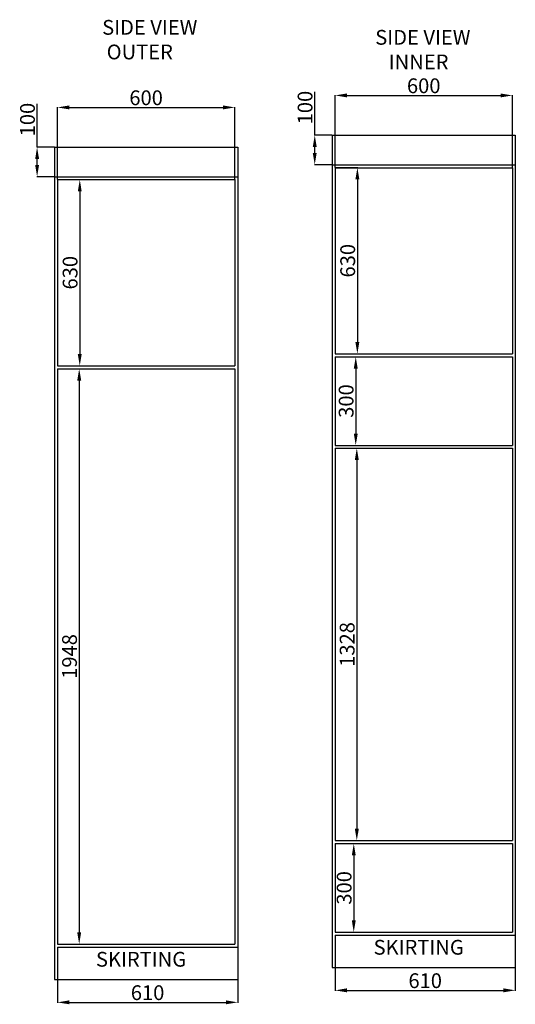
# Model space of a CAD drawing. Units: millimetres. Extents: x 46070 to 59439, y 6883 to 14761.
# Tile 4 of 5: x 56815 to 58493, y 7101 to 10434. Entities that reach past the tile are written whole.
import ezdxf

# ---------------------------------------------------------------- set-up
doc = ezdxf.new("R2010")
doc.units = ezdxf.units.MM
for name, color, linetype, lineweight in [('A-ANNO-DIMS', 2, 'Continuous', 18), ('A-ANNO-TEXT', 7, 'Continuous', 18), ('A-ELEV', 7, 'Continuous', 25)]:
    doc.layers.add(name, color=color, linetype=linetype, lineweight=lineweight)
doc.styles.get("Standard").update_dxf_attribs({"font": 'arial.ttf'})
doc.dimstyles.new('ISO-25', dxfattribs={"dimtxt": 50, "dimasz": 40, "dimexe": 1.25, "dimexo": 0.625, "dimtad": 1, "dimtxsty": 'Standard', "dimcen": 2.5, "dimadec": 0, "dimazin": 0, "dimtfac": 1, "dimtmove": 0, "dimatfit": 3, "dimfxl": 1, "dimarcsym": 0})

# ---------------------------------------------------------------- blocks, each defined once
blk = doc.blocks.new('*D68')
at = {"layer": 'A-ANNO-DIMS', "color": 0, "lineweight": -2, "transparency": 16777216}
for p, q in [((57883.3, 7644.7), (57947.2, 7644.7)), ((57945.9, 7604.7), (57945.9, 7384.7)), ((57883.3, 7344.7), (57947.2, 7344.7))]:
    blk.add_line(p, q, dxfattribs=at)
at = {"layer": 'A-ANNO-DIMS', "color": 0, "transparency": 16777216}
for points in [[(57939.3, 7604.7), (57952.6, 7604.7), (57945.9, 7644.7)], [(57939.3, 7384.7), (57952.6, 7384.7), (57945.9, 7344.7)]]:
    blk.add_solid(points, dxfattribs=at)
at = {"layer": 'Defpoints', "color": 0, "transparency": 16777216}
for p in [(57882.7, 7644.7), (57882.7, 7344.7), (57945.9, 7344.7)]:
    blk.add_point(p, dxfattribs=at)
at = {"layer": 'A-ANNO-DIMS', "color": 0, "transparency": 16777216, "insert": (57919.8, 7494.7), "char_height": 50, "attachment_point": 5, "rotation": 90}
blk.add_mtext('300', dxfattribs=at)
blk = doc.blocks.new('*D69')
at = {"layer": 'A-ANNO-DIMS', "color": 0, "lineweight": -2, "transparency": 16777216}
for p, q in [((57883.3, 8982.7), (57957.5, 8982.7)), ((57956.2, 8942.7), (57956.2, 7694.7)), ((57883.3, 7654.7), (57957.5, 7654.7))]:
    blk.add_line(p, q, dxfattribs=at)
at = {"layer": 'A-ANNO-DIMS', "color": 0, "transparency": 16777216}
for points in [[(57949.5, 8942.7), (57962.9, 8942.7), (57956.2, 8982.7)], [(57949.5, 7694.7), (57962.9, 7694.7), (57956.2, 7654.7)]]:
    blk.add_solid(points, dxfattribs=at)
at = {"layer": 'Defpoints', "color": 0, "transparency": 16777216}
for p in [(57882.7, 8982.7), (57882.7, 7654.7), (57956.2, 7654.7)]:
    blk.add_point(p, dxfattribs=at)
at = {"layer": 'A-ANNO-DIMS', "color": 0, "transparency": 16777216, "insert": (57930, 8318.7), "char_height": 50, "attachment_point": 5, "rotation": 90}
blk.add_mtext('1328', dxfattribs=at)
blk = doc.blocks.new('*D70')
at = {"layer": 'A-ANNO-DIMS', "color": 0, "lineweight": -2, "transparency": 16777216}
for p, q in [((57883.3, 9292.7), (57953.9, 9292.7)), ((57952.6, 9252.7), (57952.6, 9032.7)), ((57883.3, 8992.7), (57953.9, 8992.7))]:
    blk.add_line(p, q, dxfattribs=at)
at = {"layer": 'A-ANNO-DIMS', "color": 0, "transparency": 16777216}
for points in [[(57946, 9252.7), (57959.3, 9252.7), (57952.6, 9292.7)], [(57946, 9032.7), (57959.3, 9032.7), (57952.6, 8992.7)]]:
    blk.add_solid(points, dxfattribs=at)
at = {"layer": 'Defpoints', "color": 0, "transparency": 16777216}
for p in [(57882.7, 9292.7), (57882.7, 8992.7), (57952.6, 8992.7)]:
    blk.add_point(p, dxfattribs=at)
at = {"layer": 'A-ANNO-DIMS', "color": 0, "transparency": 16777216, "insert": (57926.5, 9142.7), "char_height": 50, "attachment_point": 5, "rotation": 90}
blk.add_mtext('300', dxfattribs=at)
blk = doc.blocks.new('*D71')
at = {"layer": 'A-ANNO-DIMS', "color": 0, "lineweight": -2, "transparency": 16777216}
for p, q in [((57883.3, 9932.7), (57959.3, 9932.7)), ((57958.1, 9892.7), (57958.1, 9342.7)), ((57883.3, 9302.7), (57959.3, 9302.7))]:
    blk.add_line(p, q, dxfattribs=at)
at = {"layer": 'A-ANNO-DIMS', "color": 0, "transparency": 16777216}
for points in [[(57951.4, 9892.7), (57964.8, 9892.7), (57958.1, 9932.7)], [(57951.4, 9342.7), (57964.8, 9342.7), (57958.1, 9302.7)]]:
    blk.add_solid(points, dxfattribs=at)
at = {"layer": 'Defpoints', "color": 0, "transparency": 16777216}
for p in [(57882.7, 9932.7), (57882.7, 9302.7), (57958.1, 9302.7)]:
    blk.add_point(p, dxfattribs=at)
at = {"layer": 'A-ANNO-DIMS', "color": 0, "transparency": 16777216, "insert": (57931.9, 9617.7), "char_height": 50, "attachment_point": 5, "rotation": 90}
blk.add_mtext('630', dxfattribs=at)
blk = doc.blocks.new('*D72')
at = {"layer": 'A-ANNO-DIMS', "color": 0, "lineweight": -2, "transparency": 16777216}
for p, q in [((57813.8, 10042.7), (57813.8, 10189.5)), ((57872.1, 10042.7), (57812.5, 10042.7)), ((57813.8, 9982.7), (57813.8, 10002.7)), ((57872.1, 9942.7), (57812.5, 9942.7))]:
    blk.add_line(p, q, dxfattribs=at)
at = {"layer": 'A-ANNO-DIMS', "color": 0, "transparency": 16777216}
for points in [[(57807.1, 10002.7), (57820.4, 10002.7), (57813.8, 10042.7)], [(57807.1, 9982.7), (57820.4, 9982.7), (57813.8, 9942.7)]]:
    blk.add_solid(points, dxfattribs=at)
at = {"layer": 'Defpoints', "color": 0, "transparency": 16777216}
for p in [(57813.8, 10042.7), (57872.7, 10042.7), (57872.7, 9942.7)]:
    blk.add_point(p, dxfattribs=at)
at = {"layer": 'A-ANNO-DIMS', "color": 0, "transparency": 16777216, "insert": (57787.6, 10136.1), "char_height": 50, "attachment_point": 5, "rotation": 90}
blk.add_mtext('100', dxfattribs=at)
blk = doc.blocks.new('*D73')
at = {"layer": 'A-ANNO-DIMS', "color": 0, "lineweight": -2, "transparency": 16777216}
for p, q in [((57882.7, 7334.1), (57882.7, 7146.6)), ((58492.7, 7334.1), (58492.7, 7146.6)), ((57922.7, 7147.8), (58452.7, 7147.8))]:
    blk.add_line(p, q, dxfattribs=at)
at = {"layer": 'A-ANNO-DIMS', "color": 0, "transparency": 16777216}
for points in [[(57922.7, 7154.5), (57922.7, 7141.2), (57882.7, 7147.8)], [(58452.7, 7154.5), (58452.7, 7141.2), (58492.7, 7147.8)]]:
    blk.add_solid(points, dxfattribs=at)
at = {"layer": 'Defpoints', "color": 0, "transparency": 16777216}
for p in [(57882.7, 7334.7), (58492.7, 7334.7), (58492.7, 7147.8)]:
    blk.add_point(p, dxfattribs=at)
at = {"layer": 'A-ANNO-DIMS', "color": 0, "transparency": 16777216, "insert": (58187.7, 7174), "char_height": 50, "attachment_point": 5}
blk.add_mtext('610', dxfattribs=at)
blk = doc.blocks.new('*D74')
at = {"layer": 'A-ANNO-DIMS', "color": 0, "lineweight": -2, "transparency": 16777216}
for p, q in [((57882.7, 9933.3), (57882.7, 10178.5)), ((57922.7, 10177.2), (58442.7, 10177.2)), ((58482.7, 9933.3), (58482.7, 10178.5))]:
    blk.add_line(p, q, dxfattribs=at)
at = {"layer": 'A-ANNO-DIMS', "color": 0, "transparency": 16777216}
for points in [[(57922.7, 10183.9), (57922.7, 10170.6), (57882.7, 10177.2)], [(58442.7, 10183.9), (58442.7, 10170.6), (58482.7, 10177.2)]]:
    blk.add_solid(points, dxfattribs=at)
at = {"layer": 'Defpoints', "color": 0, "transparency": 16777216}
for p in [(58482.7, 10177.2), (57882.7, 9932.7), (58482.7, 9932.7)]:
    blk.add_point(p, dxfattribs=at)
at = {"layer": 'A-ANNO-DIMS', "color": 0, "transparency": 16777216, "insert": (58182.7, 10203.4), "char_height": 50, "attachment_point": 5}
blk.add_mtext('600', dxfattribs=at)
blk = doc.blocks.new('*D75')
at = {"layer": 'A-ANNO-DIMS', "color": 0, "lineweight": -2, "transparency": 16777216}
for p, q in [((56943.6, 9252.1), (57017.7, 9252.1)), ((57016.5, 9212.1), (57016.5, 7344.1)), ((56943.6, 7304.1), (57017.7, 7304.1))]:
    blk.add_line(p, q, dxfattribs=at)
at = {"layer": 'A-ANNO-DIMS', "color": 0, "transparency": 16777216}
for points in [[(57009.8, 9212.1), (57023.2, 9212.1), (57016.5, 9252.1)], [(57009.8, 7344.1), (57023.2, 7344.1), (57016.5, 7304.1)]]:
    blk.add_solid(points, dxfattribs=at)
at = {"layer": 'Defpoints', "color": 0, "transparency": 16777216}
for p in [(56943, 9252.1), (56943, 7304.1), (57016.5, 7304.1)]:
    blk.add_point(p, dxfattribs=at)
at = {"layer": 'A-ANNO-DIMS', "color": 0, "transparency": 16777216, "insert": (56990.3, 8278.1), "char_height": 50, "attachment_point": 5, "rotation": 90}
blk.add_mtext('1948', dxfattribs=at)
blk = doc.blocks.new('*D76')
at = {"layer": 'A-ANNO-DIMS', "color": 0, "lineweight": -2, "transparency": 16777216}
for p, q in [((56943.6, 9892.1), (57019.6, 9892.1)), ((57018.4, 9852.1), (57018.4, 9302.1)), ((56943.6, 9262.1), (57019.6, 9262.1))]:
    blk.add_line(p, q, dxfattribs=at)
at = {"layer": 'A-ANNO-DIMS', "color": 0, "transparency": 16777216}
for points in [[(57011.7, 9852.1), (57025, 9852.1), (57018.4, 9892.1)], [(57011.7, 9302.1), (57025, 9302.1), (57018.4, 9262.1)]]:
    blk.add_solid(points, dxfattribs=at)
at = {"layer": 'Defpoints', "color": 0, "transparency": 16777216}
for p in [(56943, 9892.1), (56943, 9262.1), (57018.4, 9262.1)]:
    blk.add_point(p, dxfattribs=at)
at = {"layer": 'A-ANNO-DIMS', "color": 0, "transparency": 16777216, "insert": (56992.2, 9577.1), "char_height": 50, "attachment_point": 5, "rotation": 90}
blk.add_mtext('630', dxfattribs=at)
blk = doc.blocks.new('*D77')
at = {"layer": 'A-ANNO-DIMS', "color": 0, "lineweight": -2, "transparency": 16777216}
for p, q in [((56874, 10002.1), (56874, 10148.9)), ((56932.4, 10002.1), (56872.8, 10002.1)), ((56874, 9942.1), (56874, 9962.1)), ((56932.4, 9902.1), (56872.8, 9902.1))]:
    blk.add_line(p, q, dxfattribs=at)
at = {"layer": 'A-ANNO-DIMS', "color": 0, "transparency": 16777216}
for points in [[(56867.4, 9962.1), (56880.7, 9962.1), (56874, 10002.1)], [(56867.4, 9942.1), (56880.7, 9942.1), (56874, 9902.1)]]:
    blk.add_solid(points, dxfattribs=at)
at = {"layer": 'Defpoints', "color": 0, "transparency": 16777216}
for p in [(56874, 10002.1), (56933, 10002.1), (56933, 9902.1)]:
    blk.add_point(p, dxfattribs=at)
at = {"layer": 'A-ANNO-DIMS', "color": 0, "transparency": 16777216, "insert": (56847.9, 10095.5), "char_height": 50, "attachment_point": 5, "rotation": 90}
blk.add_mtext('100', dxfattribs=at)
blk = doc.blocks.new('*D78')
at = {"layer": 'A-ANNO-DIMS', "color": 0, "lineweight": -2, "transparency": 16777216}
for p, q in [((56943, 7293.4), (56943, 7106)), ((57553, 7293.4), (57553, 7106)), ((56983, 7107.2), (57513, 7107.2))]:
    blk.add_line(p, q, dxfattribs=at)
at = {"layer": 'A-ANNO-DIMS', "color": 0, "transparency": 16777216}
for points in [[(56983, 7113.9), (56983, 7100.6), (56943, 7107.2)], [(57513, 7113.9), (57513, 7100.6), (57553, 7107.2)]]:
    blk.add_solid(points, dxfattribs=at)
at = {"layer": 'Defpoints', "color": 0, "transparency": 16777216}
for p in [(56943, 7294.1), (57553, 7294.1), (57553, 7107.2)]:
    blk.add_point(p, dxfattribs=at)
at = {"layer": 'A-ANNO-DIMS', "color": 0, "transparency": 16777216, "insert": (57248, 7133.4), "char_height": 50, "attachment_point": 5}
blk.add_mtext('610', dxfattribs=at)
blk = doc.blocks.new('*D79')
at = {"layer": 'A-ANNO-DIMS', "color": 0, "lineweight": -2, "transparency": 16777216}
for p, q in [((56943, 9892.7), (56943, 10137.9)), ((56983, 10136.6), (57503, 10136.6)), ((57543, 9892.7), (57543, 10137.9))]:
    blk.add_line(p, q, dxfattribs=at)
at = {"layer": 'A-ANNO-DIMS', "color": 0, "transparency": 16777216}
for points in [[(56983, 10143.3), (56983, 10130), (56943, 10136.6)], [(57503, 10143.3), (57503, 10130), (57543, 10136.6)]]:
    blk.add_solid(points, dxfattribs=at)
at = {"layer": 'Defpoints', "color": 0, "transparency": 16777216}
for p in [(57543, 10136.6), (56943, 9892.1), (57543, 9892.1)]:
    blk.add_point(p, dxfattribs=at)
at = {"layer": 'A-ANNO-DIMS', "color": 0, "transparency": 16777216, "insert": (57243, 10162.8), "char_height": 50, "attachment_point": 5}
blk.add_mtext('600', dxfattribs=at)

msp = doc.modelspace()

# ---------------------------------------------------------------- linework, layer by layer
at = {"layer": 'A-ELEV'}
for p, q in [((57872.712, 10042.682), (57872.712, 7224.682)), ((57872.712, 10042.682), (58492.712, 10042.682)), ((58492.712, 10042.682), (58492.712, 7224.682)), ((56932.988, 10002.071), (57552.988, 10002.071)), ((56932.988, 10002.071), (56932.988, 7184.071)), ((57552.988, 10002.071), (57552.988, 7184.071)), ((57872.712, 9942.682), (58492.712, 9942.682)), ((57882.712, 9932.682), (57882.712, 9302.682)), ((57882.712, 9932.682), (58482.712, 9932.682)), ((58482.712, 9932.682), (58482.712, 9302.682)), ((56932.988, 9902.071), (57552.988, 9902.071)), ((56942.988, 9892.071), (57542.988, 9892.071)), ((56942.988, 9892.071), (56942.988, 9262.071)), ((57542.988, 9892.071), (57542.988, 9262.071)), ((57882.712, 9302.682), (58482.712, 9302.682)), ((57882.712, 9292.682), (58482.712, 9292.682)), ((57882.712, 9292.682), (57882.712, 8992.682)), ((58482.712, 9292.682), (58482.712, 8992.682)), ((56942.988, 9262.071), (57542.988, 9262.071)), ((56942.988, 9252.071), (57542.988, 9252.071)), ((56942.988, 9252.071), (56942.988, 7304.071)), ((57542.988, 9252.071), (57542.988, 7304.071)), ((57882.712, 8992.682), (58482.712, 8992.682)), ((57882.712, 8982.682), (58482.712, 8982.682)), ((57882.712, 8982.682), (57882.712, 7654.682)), ((58482.712, 8982.682), (58482.712, 7654.682)), ((57882.712, 7654.682), (58482.712, 7654.682)), ((57882.712, 7644.682), (58482.712, 7644.682)), ((57882.712, 7644.682), (57882.712, 7344.682)), ((58482.712, 7644.682), (58482.712, 7344.682)), ((57882.712, 7344.682), (58482.712, 7344.682)), ((57882.712, 7334.682), (58492.712, 7334.682)), ((57882.712, 7334.682), (57882.712, 7224.682)), ((56942.988, 7304.071), (57542.988, 7304.071)), ((56942.988, 7294.071), (57552.988, 7294.071)), ((56942.988, 7294.071), (56942.988, 7184.071)), ((57872.712, 7224.682), (58492.712, 7224.682)), ((56932.988, 7184.071), (57552.988, 7184.071))]:
    msp.add_line(p, q, dxfattribs=at)

# ---------------------------------------------------------------- texts
at = {"layer": 'A-ANNO-TEXT', "char_height": 50, "attachment_point": 1}
for s, insert in [(' SIDE VIEW \\P  OUTER', (57078.917, 10432.711)), ('SIDE VIEW \\P   INNER', (58018.641, 10398.833)), ('SKIRTING ', (58013.017, 7318.59)), ('SKIRTING ', (57073.293, 7277.979))]:
    msp.add_mtext_dynamic_manual_height_columns(s, width=502.17574, gutter_width=12.5, heights=[0], dxfattribs=dict(at, insert=insert))

# ---------------------------------------------------------------- dimensions: what is measured, and where the dimension line sits
at = {"layer": 'A-ANNO-DIMS'}
for base, p1, p2, picture, middle in [((58482.712, 10177.235), (57882.712, 9932.682), (58482.712, 9932.682), '*D74', (58182.712, 10203.389)), ((57542.988, 10136.624), (56942.988, 9892.071), (57542.988, 9892.071), '*D79', (57242.988, 10162.778)), ((58492.712, 7147.829), (57882.712, 7334.682), (58492.712, 7334.682), '*D73', (58187.712, 7173.982)), ((57552.988, 7107.218), (56942.988, 7294.071), (57552.988, 7294.071), '*D78', (57247.988, 7133.371))]:
    dim = msp.add_linear_dim(base=base, p1=p1, p2=p2, dimstyle='ISO-25', override={"dimclrd": 0, "dimclre": 0, "dimclrt": 0}, dxfattribs=at)
    dim.commit()
    dim.dimension.update_dxf_attribs({"geometry": picture, "text_midpoint": middle})
for base, p1, p2, picture, middle in [((57813.758, 10042.682), (57872.712, 9942.682), (57872.712, 10042.682), '*D72', (57787.604, 10136.104)), ((56874.034, 10002.071), (56932.988, 9902.071), (56932.988, 10002.071), '*D77', (56847.88, 10095.493)), ((57958.087, 9302.682), (57882.712, 9932.682), (57882.712, 9302.682), '*D71', (57931.917, 9617.682)), ((57018.363, 9262.071), (56942.988, 9892.071), (56942.988, 9262.071), '*D76', (56992.193, 9577.071)), ((57952.629, 8992.682), (57882.712, 9292.682), (57882.712, 8992.682), '*D70', (57926.458, 9142.682)), ((57016.485, 7304.071), (56942.988, 9252.071), (56942.988, 7304.071), '*D75', (56990.331, 8278.071)), ((57956.209, 7654.682), (57882.712, 8982.682), (57882.712, 7654.682), '*D69', (57930.038, 8318.682)), ((57945.925, 7344.682), (57882.712, 7644.682), (57882.712, 7344.682), '*D68', (57919.754, 7494.682))]:
    dim = msp.add_linear_dim(base=base, p1=p1, p2=p2, angle=90, dimstyle='ISO-25', override={"dimclrd": 0, "dimclre": 0, "dimclrt": 0}, dxfattribs=at)
    dim.commit()
    dim.dimension.update_dxf_attribs({"geometry": picture, "text_midpoint": middle})

doc.saveas('drawing.dxf')
